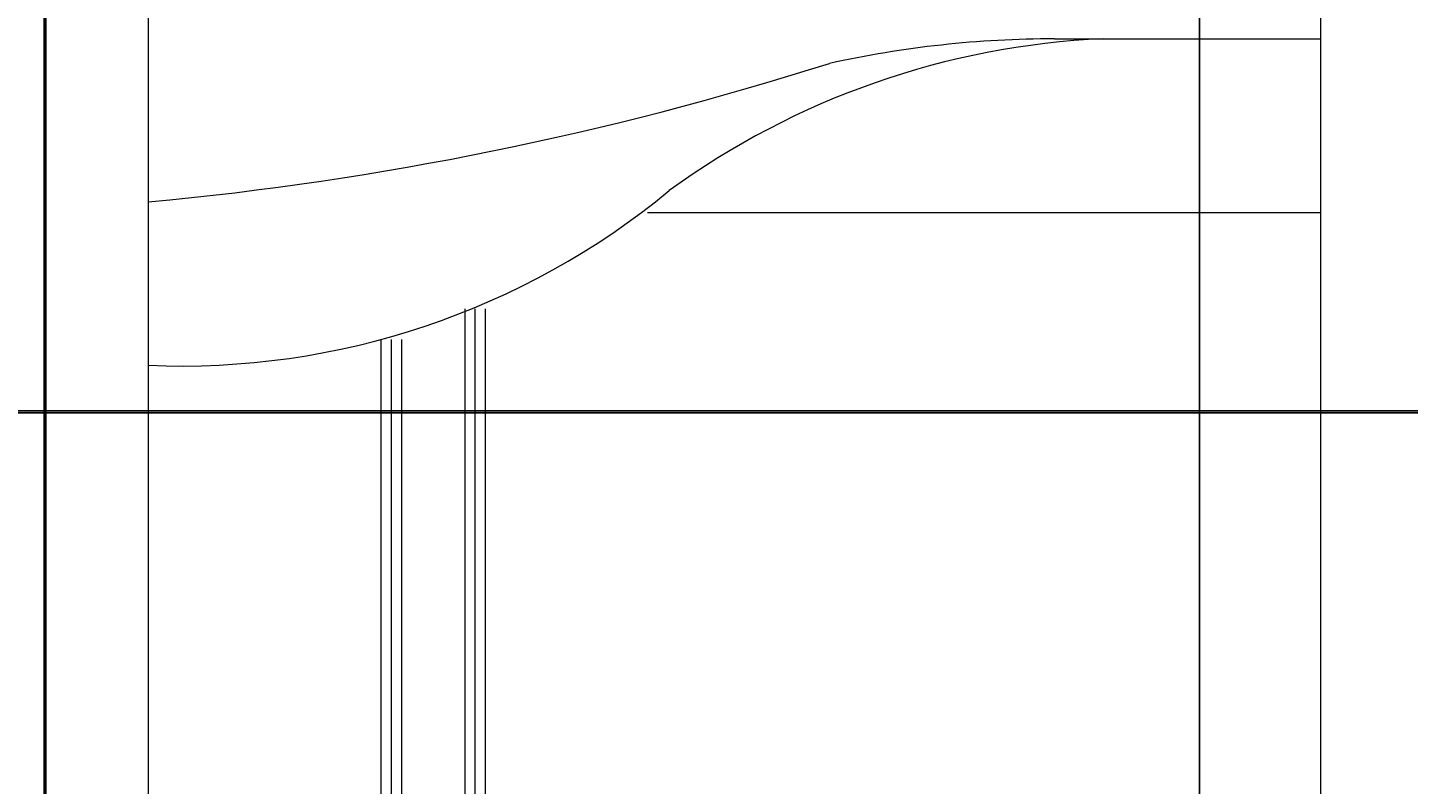
# Model space of a CAD drawing. Units: inches. Extents: x -1517 to -668, y -425 to 52.
# Tile 10 of 13: x -1186 to -1129, y -32 to -1. Entities that reach past the tile are written whole.
import ezdxf

# ---------------------------------------------------------------- set-up
doc = ezdxf.new("R2010")
doc.units = ezdxf.units.IN
doc.header["$MEASUREMENT"] = 0
for name, color, linetype, lineweight in [('A-ANNO-DIMS', 2, 'Continuous', 18), ('furniture block', 8, 'Continuous', 18), ('walls', 240, 'Continuous', 50)]:
    doc.layers.add(name, color=color, linetype=linetype, lineweight=lineweight)
doc.styles.get("Standard").update_dxf_attribs({"font": 'arial.ttf'})
doc.dimstyles.get("Standard").update_dxf_attribs({"dimtxt": 0.18, "dimasz": 0.18, "dimexe": 0.18, "dimexo": 0.0625, "dimgap": 0.09, "dimtad": 0, "dimtih": 1, "dimtoh": 1, "dimdec": 4, "dimzin": 0, "dimdsep": 46, "dimlunit": 4, "dimtxsty": 'Standard', "dimcen": 0.09, "dimadec": 0, "dimazin": 0, "dimtfac": 1, "dimtdec": 4, "dimtofl": 0, "dimtmove": 0, "dimatfit": 3, "dimfxl": 1, "dimtolj": 1, "dimtzin": 0, "dimarcsym": 0})

# ---------------------------------------------------------------- blocks, each defined once
blk = doc.blocks.new('A$C62731D1C')
for p, q in [((0.0963, 0.3882, 0.6857), (0.0963, 2.1408, 0.6857)), ((1.4679, 2.1408, 0.6857), (1.4679, 0.3882, 0.6857)), ((1.1569, 1.7598, 0.6857), (1.4679, 1.7598, 0.6857)), ((0.6805, 1.5566, 0.6857), (1.4679, 1.5566, 0.6857)), ((0.4664, 1.4437, 0.6857), (0.4664, 0.312, 0.6857)), ((0.4784, 1.4437, 0.6857), (0.4784, 0.312, 0.6857)), ((0.4904, 1.4437, 0.6857), (0.4904, 0.312, 0.6857)), ((0.3683, 1.4076, 0.6857), (0.3683, 0.312, 0.6857)), ((0.3803, 1.4076, 0.6857), (0.3803, 0.312, 0.6857)), ((0.3923, 1.4076, 0.6857), (0.3923, 0.312, 0.6857))]:
    blk.add_line(p, q)
for centre, radius, start, end in [((1.2552, 0.827, 0.6857), 0.9338, 92.5398, 126.0403), ((1.1565, 0.5405, 0.6857), 1.2193, 89.9814, 102.4667), ((-0.2581, 5.3461, 0.6857), 3.7939, 275.3572, 287.6665), ((0.1344, 2.2742, 0.6857), 0.8976, 267.5673, 309.5461)]:
    blk.add_arc(centre, radius, start, end)
blk = doc.blocks.new('A$C0E6D7E3D')
blk.add_blockref('A$C62731D1C', (0, 0))
blk = doc.blocks.new('*D36')
at = {"layer": 'A-ANNO-DIMS', "color": 0, "lineweight": -2, "transparency": 16777216}
for p, q in [((-1130.311, 17.63), (-1118.156, 17.63)), ((-1118.336, 17.45), (-1118.336, -22.314)), ((-1118.336, -62.443), (-1118.336, -22.68)), ((-1130.311, -62.623), (-1118.156, -62.623))]:
    blk.add_line(p, q, dxfattribs=at)
at = {"layer": 'A-ANNO-DIMS', "color": 0, "transparency": 16777216}
for points in [[(-1118.366, 17.45), (-1118.306, 17.45), (-1118.336, 17.63)], [(-1118.366, -62.443), (-1118.306, -62.443), (-1118.336, -62.623)]]:
    blk.add_solid(points, dxfattribs=at)
at = {"layer": 'Defpoints', "color": 0, "transparency": 16777216}
for p in [(-1130.374, 17.63), (-1118.336, 17.63), (-1130.374, -62.623)]:
    blk.add_point(p, dxfattribs=at)
at = {"layer": 'A-ANNO-DIMS', "color": 0, "transparency": 16777216, "insert": (-1118.336, -22.497), "char_height": 0.18, "attachment_point": 5}
blk.add_mtext("\\A1;CHILD'S BED 80", dxfattribs=at)
blk = doc.blocks.new('*D53')
at = {"layer": 'A-ANNO-DIMS', "color": 0, "lineweight": -2, "transparency": 16777216}
for p, q in [((-1242.504, -153.307), (-1242.504, 52.11)), ((-1014.504, -150.307), (-1014.504, 52.11)), ((-1242.324, 51.93), (-1128.794, 51.93)), ((-1014.684, 51.93), (-1128.213, 51.93))]:
    blk.add_line(p, q, dxfattribs=at)
at = {"layer": 'A-ANNO-DIMS', "color": 0, "transparency": 16777216}
for points in [[(-1242.324, 51.96), (-1242.324, 51.9), (-1242.504, 51.93)], [(-1014.684, 51.96), (-1014.684, 51.9), (-1014.504, 51.93)]]:
    blk.add_solid(points, dxfattribs=at)
at = {"layer": 'Defpoints', "color": 0, "transparency": 16777216}
for p in [(-1014.504, 51.93), (-1014.504, -150.37), (-1242.504, -153.37)]:
    blk.add_point(p, dxfattribs=at)
at = {"layer": 'A-ANNO-DIMS', "color": 0, "transparency": 16777216, "insert": (-1128.504, 51.93), "char_height": 0.18, "attachment_point": 5}
blk.add_mtext('\\A1;228', dxfattribs=at)
blk = doc.blocks.new('*D65')
at = {"layer": 'A-ANNO-DIMS', "color": 0, "lineweight": -2, "transparency": 16777216}
for p, q in [((-1138.018, -282.307), (-1138.018, 52.11)), ((-1114.018, -282.307), (-1114.018, 52.11)), ((-1137.838, 51.93), (-1126.238, 51.93)), ((-1114.198, 51.93), (-1125.798, 51.93))]:
    blk.add_line(p, q, dxfattribs=at)
at = {"layer": 'A-ANNO-DIMS', "color": 0, "transparency": 16777216}
for points in [[(-1137.838, 51.96), (-1137.838, 51.9), (-1138.018, 51.93)], [(-1114.198, 51.96), (-1114.198, 51.9), (-1114.018, 51.93)]]:
    blk.add_solid(points, dxfattribs=at)
at = {"layer": 'Defpoints', "color": 0, "transparency": 16777216}
for p in [(-1114.018, 51.93), (-1138.018, -282.37), (-1114.018, -282.37)]:
    blk.add_point(p, dxfattribs=at)
at = {"layer": 'A-ANNO-DIMS', "color": 0, "transparency": 16777216, "insert": (-1126.018, 51.93), "char_height": 0.18, "attachment_point": 5}
blk.add_mtext('\\A1;24', dxfattribs=at)
blk = doc.blocks.new('*D72')
at = {"layer": 'A-ANNO-DIMS', "color": 0, "lineweight": -2, "transparency": 16777216}
for p, q in [((-1285.841, -16.282), (-980.024, -16.282)), ((-980.204, -16.462), (-980.204, -59.144)), ((-980.204, -102.19), (-980.204, -59.508)), ((-1285.841, -102.37), (-980.024, -102.37))]:
    blk.add_line(p, q, dxfattribs=at)
at = {"layer": 'A-ANNO-DIMS', "color": 0, "transparency": 16777216}
for points in [[(-980.234, -16.462), (-980.174, -16.462), (-980.204, -16.282)], [(-980.234, -102.19), (-980.174, -102.19), (-980.204, -102.37)]]:
    blk.add_solid(points, dxfattribs=at)
at = {"layer": 'Defpoints', "color": 0, "transparency": 16777216}
for p in [(-1285.904, -16.282), (-1285.904, -102.37), (-980.204, -102.37)]:
    blk.add_point(p, dxfattribs=at)
at = {"layer": 'A-ANNO-DIMS', "color": 0, "transparency": 16777216, "insert": (-980.204, -59.326), "char_height": 0.18, "attachment_point": 5}
blk.add_mtext('\\A1;86.09', dxfattribs=at)
blk = doc.blocks.new('*D73')
at = {"layer": 'A-ANNO-DIMS', "color": 0, "lineweight": -2, "transparency": 16777216}
for p, q in [((-1089.366, -16.37), (-1516.984, -16.37)), ((-1516.804, -16.55), (-1516.804, -59.188)), ((-1516.804, -102.19), (-1516.804, -59.552)), ((-1089.366, -102.37), (-1516.984, -102.37))]:
    blk.add_line(p, q, dxfattribs=at)
at = {"layer": 'A-ANNO-DIMS', "color": 0, "transparency": 16777216}
for points in [[(-1516.834, -16.55), (-1516.774, -16.55), (-1516.804, -16.37)], [(-1516.834, -102.19), (-1516.774, -102.19), (-1516.804, -102.37)]]:
    blk.add_solid(points, dxfattribs=at)
at = {"layer": 'Defpoints', "color": 0, "transparency": 16777216}
for p in [(-1089.304, -16.37), (-1516.804, -102.37), (-1089.304, -102.37)]:
    blk.add_point(p, dxfattribs=at)
at = {"layer": 'A-ANNO-DIMS', "color": 0, "transparency": 16777216, "insert": (-1516.804, -59.37), "char_height": 0.18, "attachment_point": 5}
blk.add_mtext('\\A1;86', dxfattribs=at)

msp = doc.modelspace()

# ---------------------------------------------------------------- linework, layer by layer
at = {"layer": 'walls'}
msp.add_line((-1185.3037, -102.37), (-1185.3037, 17.63), dxfattribs=at)

# ---------------------------------------------------------------- block references
at = {"layer": 'furniture block', "xscale": 34.99562554665724, "yscale": 34.99562554665724, "zscale": 34.99562554665724}
msp.add_blockref('A$C0E6D7E3D', (-1184.4382, -62.6234), dxfattribs=at)

# ---------------------------------------------------------------- dimensions: what is measured, and where the dimension line sits
at = {"layer": 'A-ANNO-DIMS'}
for base, p1, p2, picture, middle in [((-1014.5037, 51.93), (-1242.5037, -153.37), (-1014.5037, -150.37), '*D53', (-1128.5037, 51.93)), ((-1114.0183, 51.93), (-1138.0183, -282.37), (-1114.0183, -282.37), '*D65', (-1126.0183, 51.93))]:
    dim = msp.add_linear_dim(base=base, p1=p1, p2=p2, dimstyle='Standard', override={"dimdec": 0, "dimlfac": 1, "dimrnd": 0, "dimzin": 0, "dimdsep": 46, "dimlunit": 2}, dxfattribs=at)
    dim.commit()
    dim.dimension.update_dxf_attribs({"geometry": picture, "text_midpoint": middle})
dim = msp.add_linear_dim(base=(-1118.336, 17.63), p1=(-1130.374, -62.6234), p2=(-1130.374, 17.63), angle=90, text="CHILD'S BED <>", dimstyle='Standard', override={"dimdec": 0, "dimlfac": 1, "dimrnd": 0, "dimzin": 0, "dimdsep": 46, "dimlunit": 2}, dxfattribs=at)
dim.commit()
dim.dimension.update_dxf_attribs({"geometry": '*D36', "text_midpoint": (-1118.336, -22.4967)})
for base, p1, p2, override, picture, middle in [((-1516.8037, -102.37), (-1089.3037, -16.37), (-1089.3037, -102.37), {"dimdec": 0, "dimlfac": 1, "dimrnd": 0, "dimzin": 0, "dimdsep": 46, "dimlunit": 2}, '*D73', (-1516.8037, -59.37)), ((-980.2037, -102.37), (-1285.9037, -16.2817), (-1285.9037, -102.37), {"dimdec": 2, "dimlfac": 1, "dimrnd": 0, "dimzin": 0, "dimdsep": 46, "dimlunit": 2}, '*D72', (-980.2037, -59.3258))]:
    dim = msp.add_linear_dim(base=base, p1=p1, p2=p2, angle=90, dimstyle='Standard', override=override, dxfattribs=at)
    dim.commit()
    dim.dimension.update_dxf_attribs({"geometry": picture, "text_midpoint": middle})

doc.saveas('drawing.dxf')
